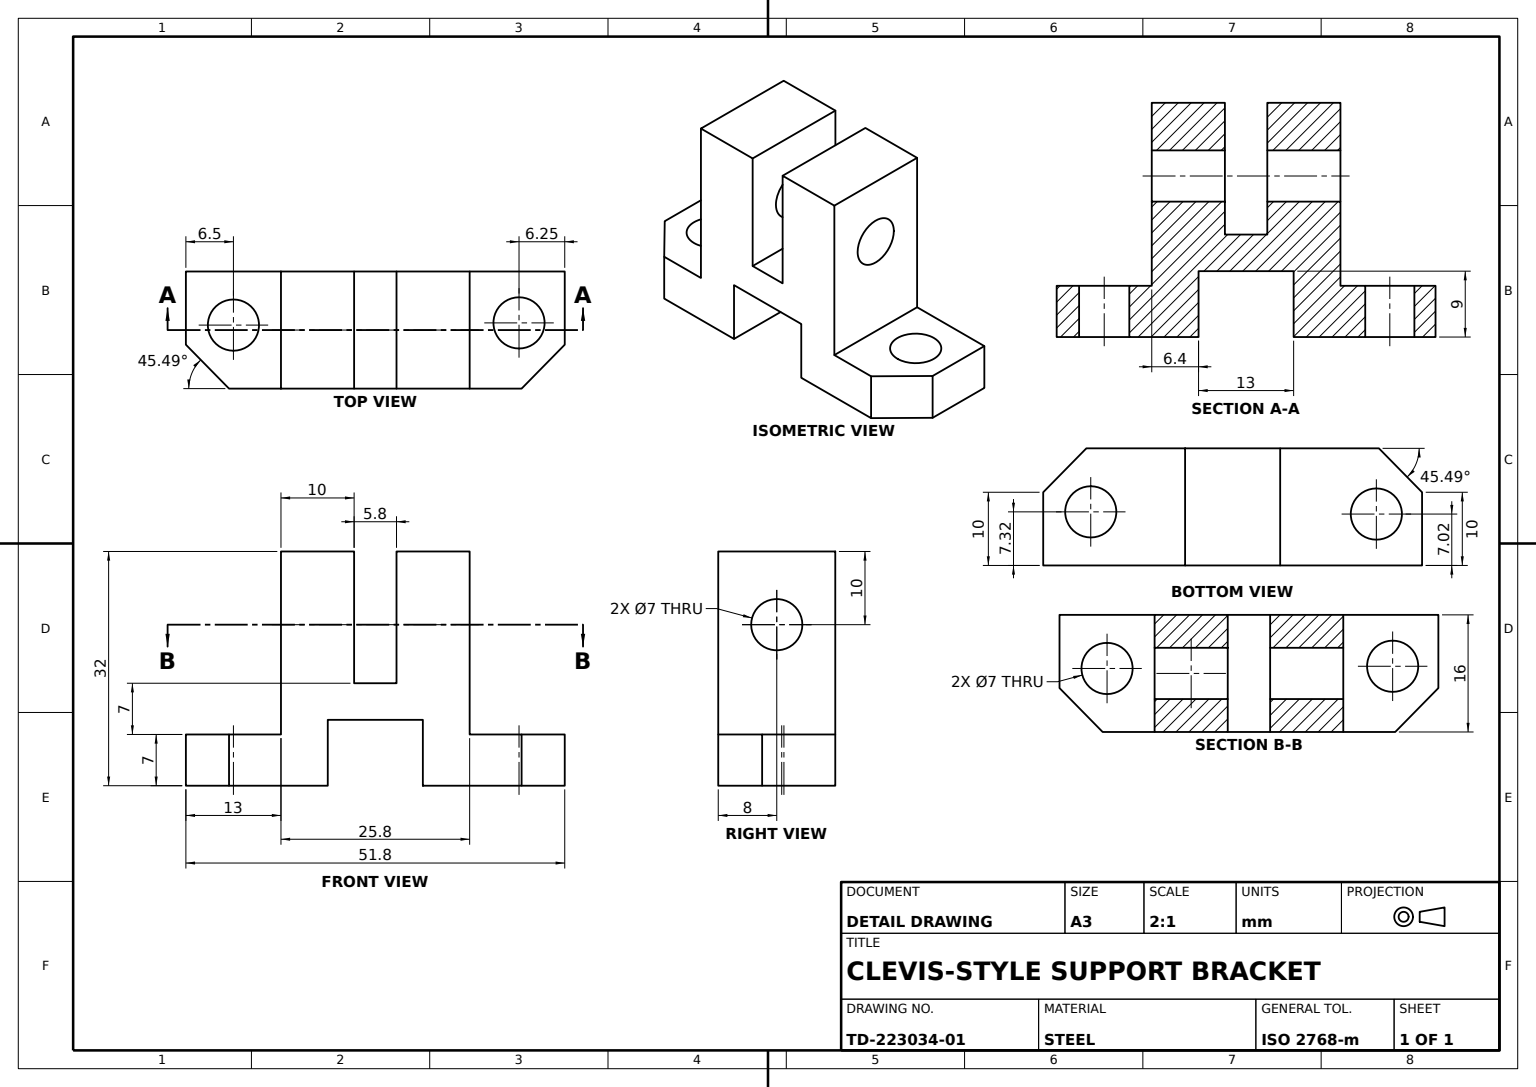
from build123d import *

# Parameters (mm, degrees)
BASE_PLATE_DEPTH              = 7
BASE_RELIEF_CUT_DEPTH         = 16
BASE_RELIEF_CUT_DEPTH_BACK    = 18
BASE_RELIEF_CUT_SKETCH_R      = 3.5
BASE_TRIM_CUT_DEPTH           = 27
BASE_TRIM_CUT_DEPTH_BACK      = 35
BASE_TRIM_CUT_SKETCH_R        = 3.5
UPRIGHT_BLOCK_SKETCH_13X13_W  = 25.796955258
UPRIGHT_BLOCK_SKETCH_13X13_H  = 16
UPRIGHT_BLOCK_DEPTH           = 25
UPRIGHT_SLOT_DEPTH            = 38
UPRIGHT_SLOT_DEPTH_BACK       = 84
UPRIGHT_CROSS_HOLE_DEPTH      = 10
UPRIGHT_CROSS_HOLE_DEPTH_BACK = 13
UPRIGHT_CROSS_HOLE_SKETCH_R   = 3.5
THROUGH_HOLE_SKETCH_R         = 3.5
THROUGH_HOLE_DEPTH            = 14
BASE_CLEARANCE_CUT_DEPTH      = 17
BASE_CLEARANCE_CUT_DEPTH_BACK = 58
BASE_CLEARANCE_CUT_SKETCH_W   = 13
BASE_CLEARANCE_CUT_SKETCH_H   = 9


with BuildPart() as part:
    # Base Plate Sketch → Base Plate (new body)
    with BuildSketch(Plane(origin=(0, 0, 0), x_dir=(1, 0, 0), z_dir=(0, 1, 0))):
        Polygon((-51.796955258, -2.197106083), (-51.796955258, -12.197106083), (-45.898477629, -18.197106083), (-5.898477629, -18.197106083), (0, -12.197106083), (0, -2.197106083), align=None)
    extrude(amount=BASE_PLATE_DEPTH)

    # Base Relief Cut Sketch → Base Relief Cut (cut, two sides: drawn at the far end of the back side and taken through both)
    with BuildSketch(Plane(origin=(0, 7, 0), x_dir=(1, 0, 0), z_dir=(0, 1, 0)).offset(-BASE_RELIEF_CUT_DEPTH_BACK)):
        with Locations(Location((-45.296955258, -9.519706742, 0), (0, 0, 270))):
            Circle(BASE_RELIEF_CUT_SKETCH_R)
    extrude(amount=BASE_RELIEF_CUT_DEPTH + BASE_RELIEF_CUT_DEPTH_BACK, mode=Mode.SUBTRACT)

    # Base Trim Cut Sketch → Base Trim Cut (cut, two sides: drawn at the far end of the back side and taken through both)
    with BuildSketch(Plane(origin=(0, 7, 0), x_dir=(1, 0, 0), z_dir=(0, 1, 0)).offset(-BASE_TRIM_CUT_DEPTH_BACK)):
        with Locations(Location((-6.250512003, -9.218640368, 0), (0, 0, 270))):
            Circle(BASE_TRIM_CUT_SKETCH_R)
    extrude(amount=BASE_TRIM_CUT_DEPTH + BASE_TRIM_CUT_DEPTH_BACK, mode=Mode.SUBTRACT)

    # Upright Block Sketch 13x13 → Upright Block (add)
    with BuildSketch(Plane(origin=(0, 7, 0), x_dir=(1, 0, 0), z_dir=(0, 1, 0))):
        with Locations((-25.898477629, -10.197106083)):
            Rectangle(UPRIGHT_BLOCK_SKETCH_13X13_W, UPRIGHT_BLOCK_SKETCH_13X13_H)
    extrude(amount=UPRIGHT_BLOCK_DEPTH)

    # Upright Slot Sketch → Upright Slot (cut, two sides: drawn at the far end of the back side and taken through both)
    with BuildSketch(Plane.XY.offset(18.197106083).offset(-UPRIGHT_SLOT_DEPTH_BACK)):
        Polygon((-28.796955258, 32), (-28.796955258, 22.247127252), (-28.796955258, 14), (-23, 14), (-23, 32), align=None)
    extrude(amount=UPRIGHT_SLOT_DEPTH + UPRIGHT_SLOT_DEPTH_BACK, mode=Mode.SUBTRACT)

    # Upright Cross Hole Sketch → Upright Cross Hole (cut, two sides: drawn at the far end of the back side and taken through both)
    with BuildSketch(Plane(origin=(-13, 0, 0), x_dir=(0, 0, -1), z_dir=(1, 0, 0)).offset(-UPRIGHT_CROSS_HOLE_DEPTH_BACK)):
        with Locations(Location((-10.197106083, 22, 0), (0, 0, 270))):
            Circle(UPRIGHT_CROSS_HOLE_SKETCH_R)
    extrude(amount=UPRIGHT_CROSS_HOLE_DEPTH + UPRIGHT_CROSS_HOLE_DEPTH_BACK, mode=Mode.SUBTRACT)

    # Through Hole Sketch → Through Hole (cut)
    with BuildSketch(Plane(origin=(-28.796955258, 0, 0), x_dir=(0, 0, -1), z_dir=(1, 0, 0))):
        with Locations(Location((-10.197106083, 22, 0), (0, 0, 270))):
            Circle(THROUGH_HOLE_SKETCH_R)
    extrude(amount=-THROUGH_HOLE_DEPTH, mode=Mode.SUBTRACT)

    # Base Clearance Cut Sketch → Base Clearance Cut (cut, two sides: drawn at the far end of the back side and taken through both)
    with BuildSketch(Plane.XY.offset(18.197106083).offset(-BASE_CLEARANCE_CUT_DEPTH_BACK)):
        with Locations((-25.898477629, 4.5)):
            Rectangle(BASE_CLEARANCE_CUT_SKETCH_W, BASE_CLEARANCE_CUT_SKETCH_H)
    extrude(amount=BASE_CLEARANCE_CUT_DEPTH + BASE_CLEARANCE_CUT_DEPTH_BACK, mode=Mode.SUBTRACT)


solid = part.part
